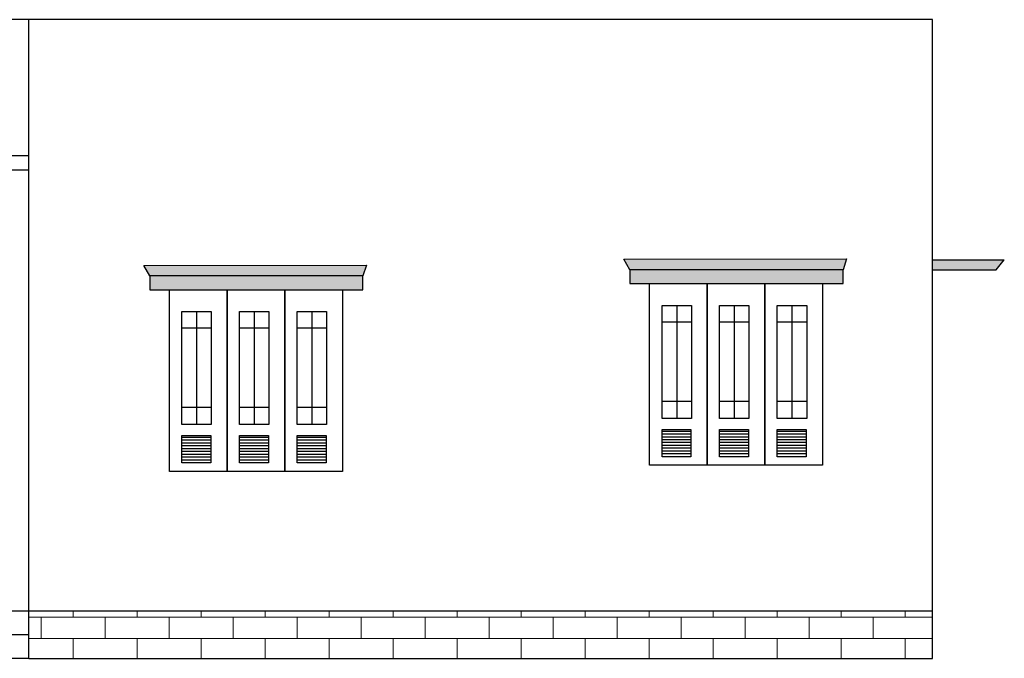
# Model space of a CAD drawing. Units: metres. Extents: x 10365 to 12529, y 3661 to 6248.
# Tile 6 of 9: x 11333 to 12379, y 4875 to 5554. Entities that reach past the tile are written whole.
import ezdxf

# ---------------------------------------------------------------- set-up
doc = ezdxf.new("R2010")
doc.units = ezdxf.units.M
doc.header["$MEASUREMENT"] = 0
doc.layers.add('A-ELEV', color=7, linetype='Continuous', lineweight=25)
doc.layers.add('A-ELEV-PATT', color=8, linetype='Continuous', lineweight=13)

msp = doc.modelspace()

# ---------------------------------------------------------------- hatches: boundary and pattern name
at = {"layer": 'A-ELEV-PATT'}
h = msp.add_hatch(color=256, dxfattribs=at)
h.dxf.hatch_style = 1
h.paths.add_polyline_path([(12208.1, 5288.4), (11981.7, 5288.4), (11981.7, 5273.7), (12208.1, 5273.7)])
h.paths.add_polyline_path([(12211.8, 5299.9), (11975.3, 5299.5), (11981.7, 5288.4), (12208.1, 5288.4)])
h = msp.add_hatch(color=256, dxfattribs=at)
h.dxf.hatch_style = 1
h.paths.add_polyline_path([(12379.5, 5299.1), (12303.2, 5299.1), (12303.2, 5288.4), (12371, 5288.4)])
h = msp.add_hatch(color=256, dxfattribs=at)
h.dxf.hatch_style = 1
h.paths.add_polyline_path([(11698, 5281.9), (11471.6, 5281.9), (11471.6, 5267.2), (11698, 5267.2)])
h.paths.add_polyline_path([(11701.7, 5293.4), (11465.1, 5293), (11471.6, 5281.9), (11698, 5281.9)])
h = msp.add_hatch(dxfattribs=at)
h.set_pattern_fill('AR-BRSTD', color=256, scale=8.5)
h.paths.add_polyline_path([(12303.2, 4925.8), (11343.2, 4925.8), (11343.2, 4875.4), (12303.2, 4875.4)])

# ---------------------------------------------------------------- linework, layer by layer
at = {"layer": 'A-ELEV'}
for p, q in [((12303.2, 5554.2), (11343.2, 5554.2)), ((11343.2, 4875.4), (11343.2, 5554.2)), ((12303.2, 4875.4), (12303.2, 5554.2)), ((10590.7, 5409.8), (11343.2, 5409.8)), ((11343.2, 5394.1), (10590.7, 5394.1)), ((11975.3, 5299.5), (12211.8, 5299.9)), ((11981.7, 5288.4), (11975.3, 5299.5)), ((12211.8, 5299.9), (12208.1, 5288.4)), ((12303.2, 5299.1), (12303.2, 5299.1)), ((12303.2, 5299.1), (12379.5, 5299.1)), ((12371, 5288.4), (12379.5, 5299.1)), ((11465.1, 5293), (11701.7, 5293.4)), ((11471.6, 5281.9), (11465.1, 5293)), ((11701.7, 5293.4), (11698, 5281.9)), ((12303.2, 5288.4), (12371, 5288.4)), ((11521.3, 5243.9), (11521.3, 5123.8)), ((11582.5, 5243.9), (11582.5, 5123.8)), ((11643.8, 5243.9), (11643.8, 5123.8)), ((12031.4, 5250.4), (12031.4, 5130.2)), ((12092.6, 5250.4), (12092.6, 5130.2)), ((12153.9, 5250.4), (12153.9, 5130.2)), ((12015.8, 5233), (12047, 5233)), ((12077, 5233), (12108.2, 5233)), ((12138.3, 5233), (12169.5, 5233)), ((11505.7, 5226.6), (11536.9, 5226.6)), ((11566.9, 5226.6), (11598.1, 5226.6)), ((11628.2, 5226.6), (11659.4, 5226.6)), ((12015.8, 5148.8), (12047, 5148.8)), ((12077, 5148.8), (12108.2, 5148.8)), ((12138.3, 5148.8), (12169.5, 5148.8)), ((11505.7, 5142.4), (11536.9, 5142.4)), ((11566.9, 5142.4), (11598.1, 5142.4)), ((11628.2, 5142.4), (11659.4, 5142.4)), ((12015.8, 5117), (12046.5, 5117)), ((12077, 5117), (12107.8, 5117)), ((12138.3, 5117), (12169, 5117)), ((11505.7, 5110.5), (11536.4, 5110.5)), ((11505.7, 5107.5), (11536.4, 5107.5)), ((11566.9, 5110.5), (11597.7, 5110.5)), ((11566.9, 5107.5), (11597.7, 5107.5)), ((11628.2, 5110.5), (11658.9, 5110.5)), ((11628.2, 5107.5), (11658.9, 5107.5)), ((12015.8, 5114), (12046.5, 5114)), ((12015.8, 5111), (12046.5, 5111)), ((12015.8, 5108), (12046.5, 5108)), ((12077, 5114), (12107.8, 5114)), ((12077, 5111), (12107.8, 5111)), ((12077, 5108), (12107.8, 5108)), ((12138.3, 5114), (12169, 5114)), ((12138.3, 5111), (12169, 5111)), ((12138.3, 5108), (12169, 5108)), ((11505.7, 5104.5), (11536.4, 5104.5)), ((11505.7, 5101.5), (11536.4, 5101.5)), ((11505.7, 5098.5), (11536.4, 5098.5)), ((11505.7, 5095.5), (11536.4, 5095.5)), ((11566.9, 5104.5), (11597.7, 5104.5)), ((11566.9, 5101.5), (11597.7, 5101.5)), ((11566.9, 5098.5), (11597.7, 5098.5)), ((11566.9, 5095.5), (11597.7, 5095.5)), ((11628.2, 5104.5), (11658.9, 5104.5)), ((11628.2, 5101.5), (11658.9, 5101.5)), ((11628.2, 5098.5), (11658.9, 5098.5)), ((11628.2, 5095.5), (11658.9, 5095.5)), ((12015.8, 5105), (12046.5, 5105)), ((12015.8, 5102), (12046.5, 5102)), ((12015.8, 5099), (12046.5, 5099)), ((12015.8, 5099), (12046.5, 5099)), ((12015.8, 5096), (12046.5, 5096)), ((12077, 5105), (12107.8, 5105)), ((12077, 5102), (12107.8, 5102)), ((12077, 5099), (12107.8, 5099)), ((12077, 5099), (12107.8, 5099)), ((12077, 5096), (12107.8, 5096)), ((12138.3, 5105), (12169, 5105)), ((12138.3, 5102), (12169, 5102)), ((12138.3, 5099), (12169, 5099)), ((12138.3, 5099), (12169, 5099)), ((12138.3, 5096), (12169, 5096)), ((11505.7, 5092.5), (11536.4, 5092.5)), ((11505.7, 5092.5), (11536.4, 5092.5)), ((11505.7, 5089.5), (11536.4, 5089.5)), ((11505.7, 5086.5), (11536.4, 5086.5)), ((11566.9, 5092.5), (11597.7, 5092.5)), ((11566.9, 5092.5), (11597.7, 5092.5)), ((11566.9, 5089.5), (11597.7, 5089.5)), ((11566.9, 5086.5), (11597.7, 5086.5)), ((11628.2, 5092.5), (11658.9, 5092.5)), ((11628.2, 5092.5), (11658.9, 5092.5)), ((11628.2, 5089.5), (11658.9, 5089.5)), ((11628.2, 5086.5), (11658.9, 5086.5)), ((12015.8, 5093), (12046.5, 5093)), ((12077, 5093), (12107.8, 5093)), ((12138.3, 5093), (12169, 5093)), ((11343.2, 4925.8), (12303.2, 4925.8)), ((11114, 4900.6), (11343.2, 4900.6)), ((11343.2, 4875.4), (10573.7, 4875.4)), ((11343.2, 4875.4), (12303.2, 4875.4))]:
    msp.add_line(p, q, dxfattribs=at)
for points in [[(11343.2, 5554.2), (11343.2, 5554.2), (10590.7, 5554.2), (10590.7, 5554.2), (10590.7, 4925.8), (10590.7, 4925.8), (11343.2, 4925.8), (11343.2, 4925.8)], [(11981.7, 5273.7), (11981.7, 5273.7), (12208.1, 5273.7), (12208.1, 5273.7), (12208.1, 5288.4), (12208.1, 5288.4), (11981.7, 5288.4), (11981.7, 5288.4)], [(11471.6, 5267.2), (11471.6, 5267.2), (11698, 5267.2), (11698, 5267.2), (11698, 5281.9), (11698, 5281.9), (11471.6, 5281.9), (11471.6, 5281.9)], [(12002.6, 5273.7), (12002.6, 5273.7), (12063.9, 5273.7), (12063.9, 5273.7), (12063.9, 5080.6), (12063.9, 5080.6), (12002.6, 5080.6), (12002.6, 5080.6)], [(12063.9, 5273.7), (12063.9, 5273.7), (12125.2, 5273.7), (12125.2, 5273.7), (12125.2, 5080.6), (12125.2, 5080.6), (12063.9, 5080.6), (12063.9, 5080.6)], [(12125.2, 5273.7), (12125.2, 5273.7), (12186.4, 5273.7), (12186.4, 5273.7), (12186.4, 5080.6), (12186.4, 5080.6), (12125.2, 5080.6), (12125.2, 5080.6)], [(11492.5, 5267.2), (11492.5, 5267.2), (11553.8, 5267.2), (11553.8, 5267.2), (11553.8, 5074.1), (11553.8, 5074.1), (11492.5, 5074.1), (11492.5, 5074.1)], [(11553.8, 5267.2), (11553.8, 5267.2), (11615.1, 5267.2), (11615.1, 5267.2), (11615.1, 5074.1), (11615.1, 5074.1), (11553.8, 5074.1), (11553.8, 5074.1)], [(11615.1, 5267.2), (11615.1, 5267.2), (11676.3, 5267.2), (11676.3, 5267.2), (11676.3, 5074.1), (11676.3, 5074.1), (11615.1, 5074.1), (11615.1, 5074.1)], [(11505.7, 5243.9), (11505.7, 5243.9), (11536.9, 5243.9), (11536.9, 5243.9), (11536.9, 5123.8), (11536.9, 5123.8), (11505.7, 5123.8), (11505.7, 5123.8)], [(11566.9, 5243.9), (11566.9, 5243.9), (11598.1, 5243.9), (11598.1, 5243.9), (11598.1, 5123.8), (11598.1, 5123.8), (11566.9, 5123.8), (11566.9, 5123.8)], [(11628.2, 5243.9), (11628.2, 5243.9), (11659.4, 5243.9), (11659.4, 5243.9), (11659.4, 5123.8), (11659.4, 5123.8), (11628.2, 5123.8), (11628.2, 5123.8)], [(12015.8, 5250.4), (12015.8, 5250.4), (12047, 5250.4), (12047, 5250.4), (12047, 5130.2), (12047, 5130.2), (12015.8, 5130.2), (12015.8, 5130.2)], [(12077, 5250.4), (12077, 5250.4), (12108.2, 5250.4), (12108.2, 5250.4), (12108.2, 5130.2), (12108.2, 5130.2), (12077, 5130.2), (12077, 5130.2)], [(12138.3, 5250.4), (12138.3, 5250.4), (12169.5, 5250.4), (12169.5, 5250.4), (12169.5, 5130.2), (12169.5, 5130.2), (12138.3, 5130.2), (12138.3, 5130.2)], [(12015.8, 5118.7), (12015.8, 5118.7), (12046.5, 5118.7), (12046.5, 5118.7), (12046.5, 5089.7), (12046.5, 5089.7), (12015.8, 5089.7), (12015.8, 5089.7)], [(12077, 5118.7), (12077, 5118.7), (12107.8, 5118.7), (12107.8, 5118.7), (12107.8, 5089.7), (12107.8, 5089.7), (12077, 5089.7), (12077, 5089.7)], [(12138.3, 5118.7), (12138.3, 5118.7), (12169, 5118.7), (12169, 5118.7), (12169, 5089.7), (12169, 5089.7), (12138.3, 5089.7), (12138.3, 5089.7)], [(11505.7, 5112.2), (11505.7, 5112.2), (11536.4, 5112.2), (11536.4, 5112.2), (11536.4, 5083.2), (11536.4, 5083.2), (11505.7, 5083.2), (11505.7, 5083.2)], [(11566.9, 5112.2), (11566.9, 5112.2), (11597.7, 5112.2), (11597.7, 5112.2), (11597.7, 5083.2), (11597.7, 5083.2), (11566.9, 5083.2), (11566.9, 5083.2)], [(11628.2, 5112.2), (11628.2, 5112.2), (11658.9, 5112.2), (11658.9, 5112.2), (11658.9, 5083.2), (11658.9, 5083.2), (11628.2, 5083.2), (11628.2, 5083.2)]]:
    msp.add_lwpolyline(points, close=True, dxfattribs=at)

doc.saveas('drawing.dxf')
